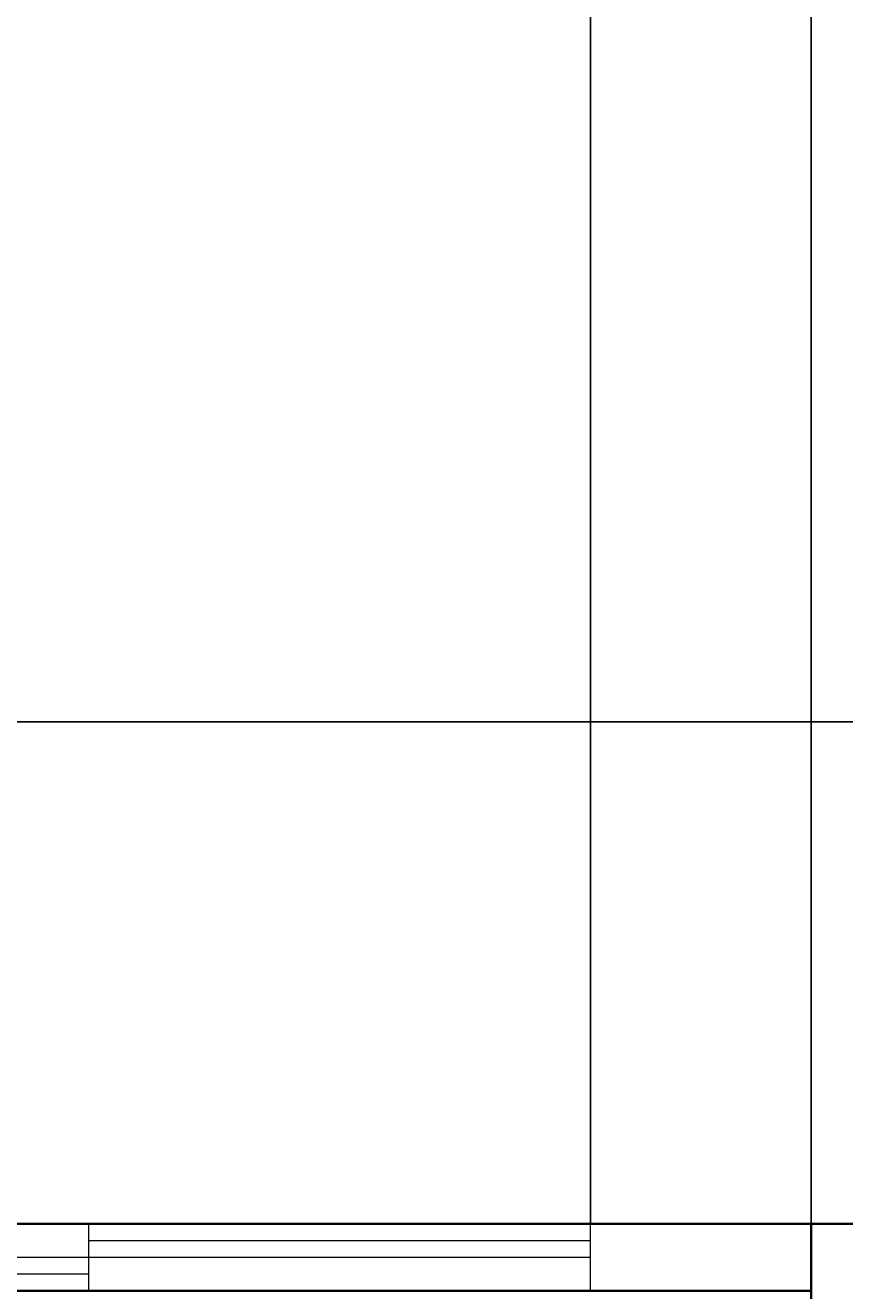
# Model space of a CAD drawing. Units: feet. Extents: x 105 to 1094, y -88 to 588.
# Tile 50 of 59: x 600 to 649, y 437 to 513. Entities that reach past the tile are written whole.
import ezdxf

# ---------------------------------------------------------------- set-up
doc = ezdxf.new("R2010")
doc.units = ezdxf.units.FT
doc.header["$MEASUREMENT"] = 0
for name, color, linetype, lineweight in [('A-ANNO-DIMS', 2, 'Continuous', 18), ('A-FLOR-PROJ', 8, 'Continuous', 25), ('A-GLAZ', 4, 'Continuous', 18), ('A-WALL', 7, 'Continuous', 35)]:
    doc.layers.add(name, color=color, linetype=linetype, lineweight=lineweight)
doc.styles.get("Standard").update_dxf_attribs({"font": 'arial.ttf'})
doc.dimstyles.get("Standard").update_dxf_attribs({"dimtxt": 0.18, "dimasz": 0.18, "dimexe": 0.18, "dimexo": 0.0625, "dimgap": 0.09, "dimtad": 0, "dimtih": 1, "dimtoh": 1, "dimdec": 4, "dimzin": 0, "dimdsep": 46, "dimtxsty": 'Standard', "dimcen": 0.09, "dimadec": 0, "dimazin": 0, "dimtfac": 1, "dimtdec": 4, "dimtofl": 0, "dimtmove": 0, "dimatfit": 3, "dimfxl": 1, "dimtolj": 1, "dimtzin": 0, "dimarcsym": 0})

# ---------------------------------------------------------------- blocks, each defined once
blk = doc.blocks.new('*D21')
at = {"layer": 'A-ANNO-DIMS', "color": 0, "lineweight": -2, "transparency": 16777216}
for p, q in [((849.626, 543.081), (105.458, 543.081)), ((105.638, 542.901), (105.638, 250.263)), ((105.638, -42.739), (105.638, 249.899)), ((849.626, -42.919), (105.458, -42.919))]:
    blk.add_line(p, q, dxfattribs=at)
at = {"layer": 'A-ANNO-DIMS', "color": 0, "transparency": 16777216}
for points in [[(105.608, 542.901), (105.668, 542.901), (105.638, 543.081)], [(105.608, -42.739), (105.668, -42.739), (105.638, -42.919)]]:
    blk.add_solid(points, dxfattribs=at)
at = {"layer": 'Defpoints', "color": 0, "transparency": 16777216}
for p in [(105.638, 543.081), (849.688, 543.081), (849.688, -42.919)]:
    blk.add_point(p, dxfattribs=at)
at = {"layer": 'A-ANNO-DIMS', "color": 0, "transparency": 16777216, "insert": (105.638, 250.081), "char_height": 0.18, "attachment_point": 5}
blk.add_mtext('\\A1;586', dxfattribs=at)
blk = doc.blocks.new('*D26')
at = {"layer": 'A-ANNO-DIMS', "color": 0, "lineweight": -2, "transparency": 16777216}
for p, q in [((552.688, 471.144), (552.688, 588.311)), ((646.688, 471.144), (646.688, 588.311)), ((552.868, 588.131), (599.47, 588.131)), ((646.508, 588.131), (599.907, 588.131))]:
    blk.add_line(p, q, dxfattribs=at)
at = {"layer": 'A-ANNO-DIMS', "color": 0, "transparency": 16777216}
for points in [[(552.868, 588.161), (552.868, 588.101), (552.688, 588.131)], [(646.508, 588.161), (646.508, 588.101), (646.688, 588.131)]]:
    blk.add_solid(points, dxfattribs=at)
at = {"layer": 'Defpoints', "color": 0, "transparency": 16777216}
for p in [(646.688, 588.131), (552.688, 471.081), (646.688, 471.081)]:
    blk.add_point(p, dxfattribs=at)
at = {"layer": 'A-ANNO-DIMS', "color": 0, "transparency": 16777216, "insert": (599.688, 588.131), "char_height": 0.18, "attachment_point": 5}
blk.add_mtext('\\A1;94', dxfattribs=at)
blk = doc.blocks.new('*D31')
at = {"layer": 'A-ANNO-DIMS', "color": 0, "lineweight": -2, "transparency": 16777216}
for p, q in [((438.751, 527.081), (1093.918, 527.081)), ((1093.738, 526.901), (1093.738, 499.263)), ((1093.738, 471.261), (1093.738, 498.899)), ((438.751, 471.081), (1093.918, 471.081))]:
    blk.add_line(p, q, dxfattribs=at)
at = {"layer": 'A-ANNO-DIMS', "color": 0, "transparency": 16777216}
for points in [[(1093.708, 526.901), (1093.768, 526.901), (1093.738, 527.081)], [(1093.708, 471.261), (1093.768, 471.261), (1093.738, 471.081)]]:
    blk.add_solid(points, dxfattribs=at)
at = {"layer": 'Defpoints', "color": 0, "transparency": 16777216}
for p in [(438.688, 527.081), (1093.738, 527.081), (438.688, 471.081)]:
    blk.add_point(p, dxfattribs=at)
at = {"layer": 'A-ANNO-DIMS', "color": 0, "transparency": 16777216, "insert": (1093.738, 499.081), "char_height": 0.18, "attachment_point": 5}
blk.add_mtext('\\A1;56', dxfattribs=at)
blk = doc.blocks.new('*D32')
at = {"layer": 'A-ANNO-DIMS', "color": 0, "lineweight": -2, "transparency": 16777216}
for p, q in [((646.626, 471.081), (105.458, 471.081)), ((105.638, 470.901), (105.638, 456.263)), ((105.638, 441.261), (105.638, 455.899)), ((646.626, 441.081), (105.458, 441.081))]:
    blk.add_line(p, q, dxfattribs=at)
at = {"layer": 'A-ANNO-DIMS', "color": 0, "transparency": 16777216}
for points in [[(105.608, 470.901), (105.668, 470.901), (105.638, 471.081)], [(105.608, 441.261), (105.668, 441.261), (105.638, 441.081)]]:
    blk.add_solid(points, dxfattribs=at)
at = {"layer": 'Defpoints', "color": 0, "transparency": 16777216}
for p in [(105.638, 471.081), (646.688, 471.081), (646.688, 441.081)]:
    blk.add_point(p, dxfattribs=at)
at = {"layer": 'A-ANNO-DIMS', "color": 0, "transparency": 16777216, "insert": (105.638, 456.081), "char_height": 0.18, "attachment_point": 5}
blk.add_mtext('\\A1;30', dxfattribs=at)
blk = doc.blocks.new('*D41')
at = {"layer": 'A-ANNO-DIMS', "color": 0, "lineweight": -2, "transparency": 16777216}
for p, q in [((646.688, 441.144), (646.688, 588.311)), ((671.688, 441.144), (671.688, 588.311)), ((646.868, 588.131), (658.967, 588.131)), ((671.508, 588.131), (659.409, 588.131))]:
    blk.add_line(p, q, dxfattribs=at)
at = {"layer": 'A-ANNO-DIMS', "color": 0, "transparency": 16777216}
for points in [[(646.868, 588.161), (646.868, 588.101), (646.688, 588.131)], [(671.508, 588.161), (671.508, 588.101), (671.688, 588.131)]]:
    blk.add_solid(points, dxfattribs=at)
at = {"layer": 'Defpoints', "color": 0, "transparency": 16777216}
for p in [(671.688, 588.131), (646.688, 441.081), (671.688, 441.081)]:
    blk.add_point(p, dxfattribs=at)
at = {"layer": 'A-ANNO-DIMS', "color": 0, "transparency": 16777216, "insert": (659.188, 588.131), "char_height": 0.18, "attachment_point": 5}
blk.add_mtext('\\A1;25', dxfattribs=at)
blk = doc.blocks.new('*D48')
at = {"layer": 'A-ANNO-DIMS', "color": 0, "lineweight": -2, "transparency": 16777216}
for p, q in [((573.483, 441.144), (573.483, 588.311)), ((633.483, 441.144), (633.483, 588.311)), ((573.663, 588.131), (603.263, 588.131)), ((633.303, 588.131), (603.702, 588.131))]:
    blk.add_line(p, q, dxfattribs=at)
at = {"layer": 'A-ANNO-DIMS', "color": 0, "transparency": 16777216}
for points in [[(573.663, 588.161), (573.663, 588.101), (573.483, 588.131)], [(633.303, 588.161), (633.303, 588.101), (633.483, 588.131)]]:
    blk.add_solid(points, dxfattribs=at)
at = {"layer": 'Defpoints', "color": 0, "transparency": 16777216}
for p in [(633.483, 588.131), (573.483, 441.081), (633.483, 441.081)]:
    blk.add_point(p, dxfattribs=at)
at = {"layer": 'A-ANNO-DIMS', "color": 0, "transparency": 16777216, "insert": (603.483, 588.131), "char_height": 0.18, "attachment_point": 5}
blk.add_mtext('\\A1;60', dxfattribs=at)

msp = doc.modelspace()

# ---------------------------------------------------------------- linework, layer by layer
at = {"layer": 'A-FLOR-PROJ'}
for p, q in [((760.6883, 471.0812), (646.6883, 471.0812)), ((646.6883, 471.0812), (646.6883, 441.0812))]:
    msp.add_line(p, q, dxfattribs=at)
at = {"layer": 'A-GLAZ'}
for p, q in [((603.4826, 437.0812), (603.4826, 441.0812)), ((633.4826, 437.0812), (633.4826, 441.0812)), ((603.4826, 440.0812), (633.4826, 440.0812)), ((603.4826, 440.0812), (633.4826, 440.0812)), ((573.4826, 439.0812), (633.4826, 439.0812)), ((573.4826, 438.0812), (603.4826, 438.0812))]:
    msp.add_line(p, q, dxfattribs=at)
at = {"layer": 'A-WALL'}
for p, q in [((646.6883, 441.0812), (552.6883, 441.0812)), ((646.6883, 441.0812), (646.6883, 288.0812)), ((760.6883, 441.0812), (646.6883, 441.0812)), ((552.6883, 437.0812), (602.6883, 437.0812)), ((602.6883, 437.0812), (646.6883, 437.0812))]:
    msp.add_line(p, q, dxfattribs=at)

# ---------------------------------------------------------------- dimensions: what is measured, and where the dimension line sits
at = {"layer": 'A-ANNO-DIMS'}
for base, p1, p2, picture, middle in [((646.6883, 588.1312), (552.6883, 471.0812), (646.6883, 471.0812), '*D26', (599.6883, 588.1312)), ((633.4826, 588.1312), (573.4826, 441.0812), (633.4826, 441.0812), '*D48', (603.4826, 588.1312)), ((671.6883, 588.1312), (646.6883, 441.0812), (671.6883, 441.0812), '*D41', (659.1883, 588.1312))]:
    dim = msp.add_linear_dim(base=base, p1=p1, p2=p2, dimstyle='Standard', override={"dimdec": 0, "dimlfac": 1, "dimrnd": 0, "dimzin": 0, "dimdsep": 46, "dimlunit": 2}, dxfattribs=at)
    dim.commit()
    dim.dimension.update_dxf_attribs({"geometry": picture, "text_midpoint": middle})
for base, p1, p2, picture, middle in [((105.6383, 543.0812), (849.6883, -42.9188), (849.6883, 543.0812), '*D21', (105.6383, 250.0812)), ((1093.7383, 527.0812), (438.6883, 471.0812), (438.6883, 527.0812), '*D31', (1093.7383, 499.0812)), ((105.6383, 471.0812), (646.6883, 441.0812), (646.6883, 471.0812), '*D32', (105.6383, 456.0812))]:
    dim = msp.add_linear_dim(base=base, p1=p1, p2=p2, angle=90, dimstyle='Standard', override={"dimdec": 0, "dimlfac": 1, "dimrnd": 0, "dimzin": 0, "dimdsep": 46, "dimlunit": 2}, dxfattribs=at)
    dim.commit()
    dim.dimension.update_dxf_attribs({"geometry": picture, "text_midpoint": middle})

doc.saveas('drawing.dxf')
